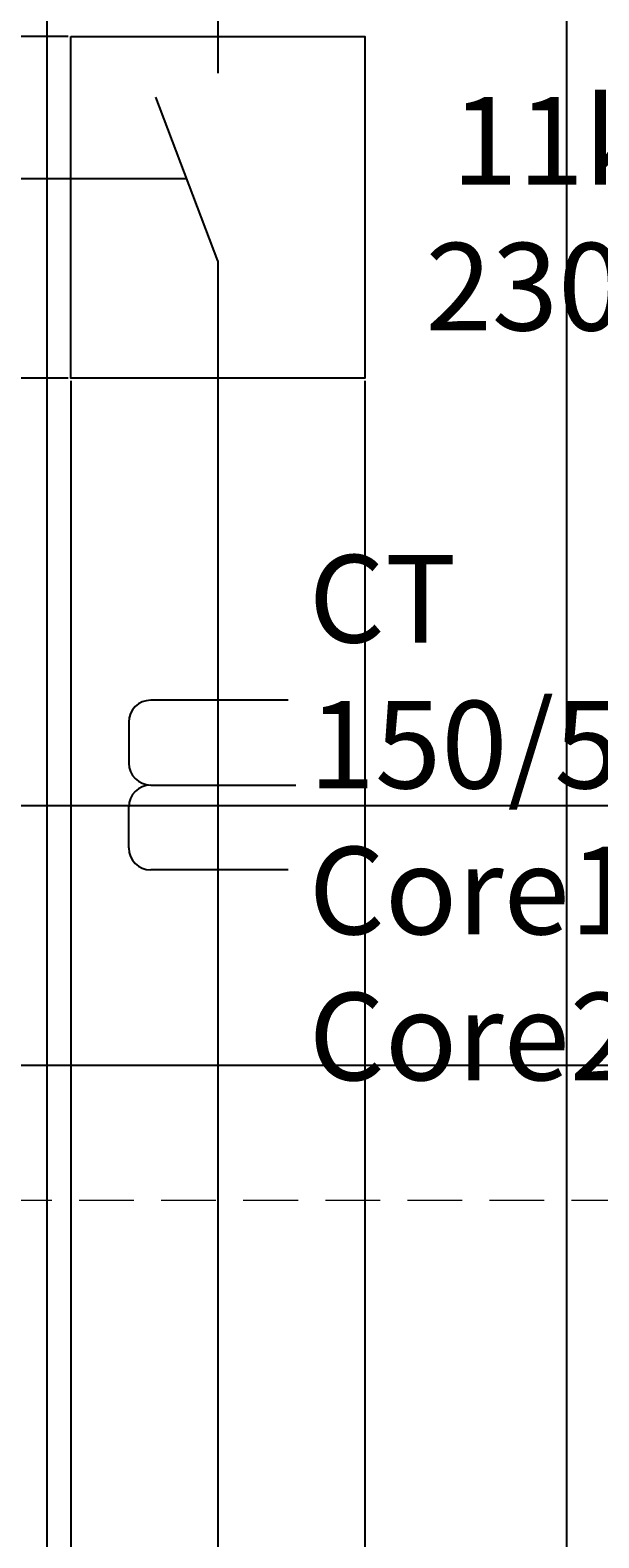
# Model space of a CAD drawing. Units: inches. Extents: x 412 to 584, y 208 to 437.
# Tile 20 of 28: x 495 to 508, y 352 to 387. Entities that reach past the tile are written whole.
import ezdxf

# ---------------------------------------------------------------- set-up
doc = ezdxf.new("R2010")
doc.units = ezdxf.units.IN
doc.header["$MEASUREMENT"] = 0
doc.linetypes.add('HIDDEN', pattern=[0.375, 0.25, -0.125])
for name, color, linetype, lineweight in [('A-ANNO-DIMS', 2, 'Continuous', 18), ('E-ANNO-TEXT', 7, 'Continuous', 18), ('E-ENCL-HIDN', 3, 'HIDDEN', 18), ('E-POWR-EQPM', 3, 'Continuous', 25)]:
    doc.layers.add(name, color=color, linetype=linetype, lineweight=lineweight)
doc.styles.get("Standard").update_dxf_attribs({"font": 'arial.ttf'})
doc.dimstyles.get("Standard").update_dxf_attribs({"dimtxt": 0.18, "dimasz": 0.18, "dimexe": 0.18, "dimexo": 0.0625, "dimgap": 0.09, "dimtad": 0, "dimtih": 1, "dimtoh": 1, "dimdec": 4, "dimzin": 0, "dimdsep": 46, "dimtxsty": 'Standard', "dimcen": 0.09, "dimadec": 0, "dimazin": 0, "dimtfac": 1, "dimtdec": 4, "dimtofl": 0, "dimtmove": 0, "dimatfit": 3, "dimfxl": 1, "dimtolj": 1, "dimtzin": 0, "dimarcsym": 0})

# ---------------------------------------------------------------- blocks, each defined once
blk = doc.blocks.new('CT-SYMBOL')
for p, q in [((3.642, 3.875), (0.5, 3.875)), ((0, 3.375), (0, 2.438)), ((0.5, 1.938), (3.819, 1.938)), ((0, 0.5), (0, 1.438)), ((3.642, 0), (0.5, 0))]:
    blk.add_line(p, q)
for centre, start, end in [((0.5, 3.375), 90, 180), ((0.5, 2.438), 180, 270), ((0.5, 1.438), 90, 180), ((0.5, 0.5), 180, 270)]:
    blk.add_arc(centre, 0.5, start, end)
blk = doc.blocks.new('*D17')
at = {"layer": 'A-ANNO-DIMS', "color": 0, "lineweight": -2, "transparency": 16777216}
for p, q in [((497.715, 426.185), (583.674, 426.185)), ((583.494, 426.005), (583.494, 323.031)), ((583.494, 219.693), (583.494, 322.667)), ((550.198, 219.513), (583.674, 219.513))]:
    blk.add_line(p, q, dxfattribs=at)
at = {"layer": 'A-ANNO-DIMS', "color": 0, "transparency": 16777216}
for points in [[(583.464, 426.005), (583.524, 426.005), (583.494, 426.185)], [(583.464, 219.693), (583.524, 219.693), (583.494, 219.513)]]:
    blk.add_solid(points, dxfattribs=at)
at = {"layer": 'Defpoints', "color": 0, "transparency": 16777216}
for p in [(497.652, 426.185), (550.135, 219.513), (583.494, 219.513)]:
    blk.add_point(p, dxfattribs=at)
at = {"layer": 'A-ANNO-DIMS', "color": 0, "transparency": 16777216, "insert": (583.494, 322.849), "char_height": 0.18, "attachment_point": 5}
blk.add_mtext('\\A1;206.67', dxfattribs=at)
blk = doc.blocks.new('*D23')
at = {"layer": 'A-ANNO-DIMS', "color": 0, "lineweight": -2, "transparency": 16777216}
for p, q in [((466.041, 360.196), (412.276, 360.196)), ((412.456, 360.016), (412.456, 354.967)), ((412.456, 349.553), (412.456, 354.603)), ((499.225, 349.373), (412.276, 349.373))]:
    blk.add_line(p, q, dxfattribs=at)
at = {"layer": 'A-ANNO-DIMS', "color": 0, "transparency": 16777216}
for points in [[(412.426, 360.016), (412.486, 360.016), (412.456, 360.196)], [(412.426, 349.553), (412.486, 349.553), (412.456, 349.373)]]:
    blk.add_solid(points, dxfattribs=at)
at = {"layer": 'Defpoints', "color": 0, "transparency": 16777216}
for p in [(466.104, 360.196), (412.456, 349.373), (499.288, 349.373)]:
    blk.add_point(p, dxfattribs=at)
at = {"layer": 'A-ANNO-DIMS', "color": 0, "transparency": 16777216, "insert": (412.456, 354.785), "char_height": 0.18, "attachment_point": 5}
blk.add_mtext('\\A1;10.823', dxfattribs=at)
blk = doc.blocks.new('*D28')
at = {"layer": 'A-ANNO-DIMS', "color": 0, "lineweight": -2, "transparency": 16777216}
for p, q in [((450.562, 256.635), (450.562, 437.465)), ((450.742, 437.285), (502.724, 437.285)), ((555.616, 437.285), (503.634, 437.285)), ((555.796, 256.635), (555.796, 437.465))]:
    blk.add_line(p, q, dxfattribs=at)
at = {"layer": 'A-ANNO-DIMS', "color": 0, "transparency": 16777216}
for points in [[(450.742, 437.315), (450.742, 437.255), (450.562, 437.285)], [(555.616, 437.315), (555.616, 437.255), (555.796, 437.285)]]:
    blk.add_solid(points, dxfattribs=at)
at = {"layer": 'Defpoints', "color": 0, "transparency": 16777216}
for p in [(555.796, 437.285), (450.562, 256.573), (555.796, 256.573)]:
    blk.add_point(p, dxfattribs=at)
at = {"layer": 'A-ANNO-DIMS', "color": 0, "transparency": 16777216, "insert": (503.179, 437.285), "char_height": 0.18, "attachment_point": 5}
blk.add_mtext('\\A1;105.23', dxfattribs=at)
blk = doc.blocks.new('*D29')
at = {"layer": 'A-ANNO-DIMS', "color": 0, "lineweight": -2, "transparency": 16777216}
for p, q in [((495.927, 378.924), (495.927, 208.233)), ((502.649, 378.924), (502.649, 208.233)), ((496.107, 208.413), (498.895, 208.413)), ((502.469, 208.413), (499.681, 208.413))]:
    blk.add_line(p, q, dxfattribs=at)
at = {"layer": 'A-ANNO-DIMS', "color": 0, "transparency": 16777216}
for points in [[(496.107, 208.443), (496.107, 208.383), (495.927, 208.413)], [(502.469, 208.443), (502.469, 208.383), (502.649, 208.413)]]:
    blk.add_solid(points, dxfattribs=at)
at = {"layer": 'Defpoints', "color": 0, "transparency": 16777216}
for p in [(495.927, 378.987), (502.649, 378.987), (502.649, 208.413)]:
    blk.add_point(p, dxfattribs=at)
at = {"layer": 'A-ANNO-DIMS', "color": 0, "transparency": 16777216, "insert": (499.288, 208.413), "char_height": 0.18, "attachment_point": 5}
blk.add_mtext('\\A1;6.722', dxfattribs=at)
blk = doc.blocks.new('*D30')
at = {"layer": 'A-ANNO-DIMS', "color": 0, "lineweight": -2, "transparency": 16777216}
for p, q in [((495.864, 386.793), (412.276, 386.793)), ((412.456, 386.613), (412.456, 383.072)), ((412.456, 379.167), (412.456, 382.708)), ((495.864, 378.987), (412.276, 378.987))]:
    blk.add_line(p, q, dxfattribs=at)
at = {"layer": 'A-ANNO-DIMS', "color": 0, "transparency": 16777216}
for points in [[(412.426, 386.613), (412.486, 386.613), (412.456, 386.793)], [(412.426, 379.167), (412.486, 379.167), (412.456, 378.987)]]:
    blk.add_solid(points, dxfattribs=at)
at = {"layer": 'Defpoints', "color": 0, "transparency": 16777216}
for p in [(495.927, 386.793), (412.456, 378.987), (495.927, 378.987)]:
    blk.add_point(p, dxfattribs=at)
at = {"layer": 'A-ANNO-DIMS', "color": 0, "transparency": 16777216, "insert": (412.456, 382.89), "char_height": 0.18, "attachment_point": 5}
blk.add_mtext('\\A1;7.807', dxfattribs=at)
blk = doc.blocks.new('*D31')
at = {"layer": 'A-ANNO-DIMS', "color": 0, "lineweight": -2, "transparency": 16777216}
for p, q in [((495.375, 405.385), (495.375, 208.233)), ((507.254, 405.385), (507.254, 208.233)), ((495.555, 208.413), (500.929, 208.413)), ((507.074, 208.413), (501.7, 208.413))]:
    blk.add_line(p, q, dxfattribs=at)
at = {"layer": 'A-ANNO-DIMS', "color": 0, "transparency": 16777216}
for points in [[(495.555, 208.443), (495.555, 208.383), (495.375, 208.413)], [(507.074, 208.443), (507.074, 208.383), (507.254, 208.413)]]:
    blk.add_solid(points, dxfattribs=at)
at = {"layer": 'Defpoints', "color": 0, "transparency": 16777216}
for p in [(495.375, 405.448), (507.254, 405.448), (507.254, 208.413)]:
    blk.add_point(p, dxfattribs=at)
at = {"layer": 'A-ANNO-DIMS', "color": 0, "transparency": 16777216, "insert": (501.314, 208.413), "char_height": 0.18, "attachment_point": 5}
blk.add_mtext('\\A1;11.88', dxfattribs=at)
blk = doc.blocks.new('*D35')
at = {"layer": 'A-ANNO-DIMS', "color": 0, "lineweight": -2, "transparency": 16777216}
for p, q in [((485.523, 369.221), (583.674, 369.221)), ((583.494, 369.041), (583.494, 366.437)), ((583.494, 363.469), (583.494, 366.073)), ((485.523, 363.289), (583.674, 363.289))]:
    blk.add_line(p, q, dxfattribs=at)
at = {"layer": 'A-ANNO-DIMS', "color": 0, "transparency": 16777216}
for points in [[(583.464, 369.041), (583.524, 369.041), (583.494, 369.221)], [(583.464, 363.469), (583.524, 363.469), (583.494, 363.289)]]:
    blk.add_solid(points, dxfattribs=at)
at = {"layer": 'Defpoints', "color": 0, "transparency": 16777216}
for p in [(485.46, 369.221), (485.46, 363.289), (583.494, 363.289)]:
    blk.add_point(p, dxfattribs=at)
at = {"layer": 'A-ANNO-DIMS', "color": 0, "transparency": 16777216, "insert": (583.494, 366.255), "char_height": 0.18, "attachment_point": 5}
blk.add_mtext('\\A1;5.932', dxfattribs=at)

msp = doc.modelspace()

# ---------------------------------------------------------------- linework, layer by layer
at = {"layer": 'E-ENCL-HIDN', "ltscale": 5}
msp.add_lwpolyline([(466.1037, 400.175), (538.6186, 400.175), (538.6186, 360.1961), (466.1037, 360.1961)], close=True, dxfattribs=at)
at = {"layer": 'E-POWR-EQPM'}
for p, q in [((499.2878, 397.3692), (499.2878, 385.9599)), ((499.2878, 381.671), (497.8672, 385.4054)), ((498.5775, 383.5382), (490.5891, 383.5382)), ((499.2878, 381.671), (499.2878, 358.9229)), ((499.2878, 358.9229), (499.2878, 349.3734))]:
    msp.add_line(p, q, dxfattribs=at)
msp.add_lwpolyline([(495.9268, 386.7933), (502.6489, 386.7933), (502.6489, 378.9867), (495.9268, 378.9867)], close=True, dxfattribs=at)

# ---------------------------------------------------------------- block references
msp.add_blockref('CT-SYMBOL', (497.252, 367.753), dxfattribs=at)

# ---------------------------------------------------------------- texts
at = {"layer": 'E-ANNO-TEXT', "char_height": 2, "attachment_point": 1}
for s, width, heights, insert in [('\\pxqc;11kV VCB\\P230A 25kA', 15.674937, [6.8044], (502.7, 385.4105)), ('\\pxql;CT\\P150/5/5A\\PCore1: 1VA, CL 0.5M5\\PCore2: 15VA, CL 10P10', 41.457397, [15.3449], (501.3634, 374.947))]:
    msp.add_mtext_dynamic_manual_height_columns(s, width=width, gutter_width=1, heights=heights, dxfattribs=dict(at, insert=insert))

# ---------------------------------------------------------------- dimensions: what is measured, and where the dimension line sits
at = {"layer": 'A-ANNO-DIMS'}
for base, p1, p2, override, picture, middle in [((555.7959, 437.2847), (450.562, 256.5729), (555.7959, 256.5729), {"dimdec": 2, "dimlfac": 1, "dimrnd": 0, "dimzin": 0, "dimdsep": 46, "dimlunit": 2}, '*D28', (503.1789, 437.2847)), ((507.2538, 208.4133), (495.3746, 405.448), (507.2538, 405.448), {"dimdec": 2, "dimlfac": 1, "dimrnd": 0, "dimzin": 0, "dimdsep": 46, "dimlunit": 2}, '*D31', (501.3142, 208.4133)), ((502.6489, 208.4133), (495.9268, 378.9867), (502.6489, 378.9867), {"dimdec": 3, "dimlfac": 1, "dimrnd": 0, "dimzin": 0, "dimdsep": 46, "dimlunit": 2}, '*D29', (499.2878, 208.4133))]:
    dim = msp.add_linear_dim(base=base, p1=p1, p2=p2, dimstyle='Standard', override=override, dxfattribs=at)
    dim.commit()
    dim.dimension.update_dxf_attribs({"geometry": picture, "text_midpoint": middle})
for base, p1, p2, override, picture, middle in [((583.4937, 219.5133), (497.6523, 426.1847), (550.1351, 219.5133), {"dimdec": 2, "dimlfac": 1, "dimrnd": 0, "dimzin": 0, "dimdsep": 46, "dimlunit": 2}, '*D17', (583.4937, 322.849)), ((412.4562, 378.9867), (495.9268, 386.7933), (495.9268, 378.9867), {"dimdec": 3, "dimlfac": 1, "dimrnd": 0, "dimzin": 0, "dimdsep": 46, "dimlunit": 2}, '*D30', (412.4562, 382.89)), ((583.4937, 363.2888), (485.4605, 369.221), (485.4605, 363.2888), {"dimdec": 3, "dimlfac": 1, "dimrnd": 0, "dimzin": 0, "dimdsep": 46, "dimlunit": 2}, '*D35', (583.4937, 366.2549)), ((412.4562, 349.3734), (466.1037, 360.1961), (499.2878, 349.3734), {"dimdec": 3, "dimlfac": 1, "dimrnd": 0, "dimzin": 0, "dimdsep": 46, "dimlunit": 2}, '*D23', (412.4562, 354.7847))]:
    dim = msp.add_linear_dim(base=base, p1=p1, p2=p2, angle=90, dimstyle='Standard', override=override, dxfattribs=at)
    dim.commit()
    dim.dimension.update_dxf_attribs({"geometry": picture, "text_midpoint": middle})

doc.saveas('drawing.dxf')
